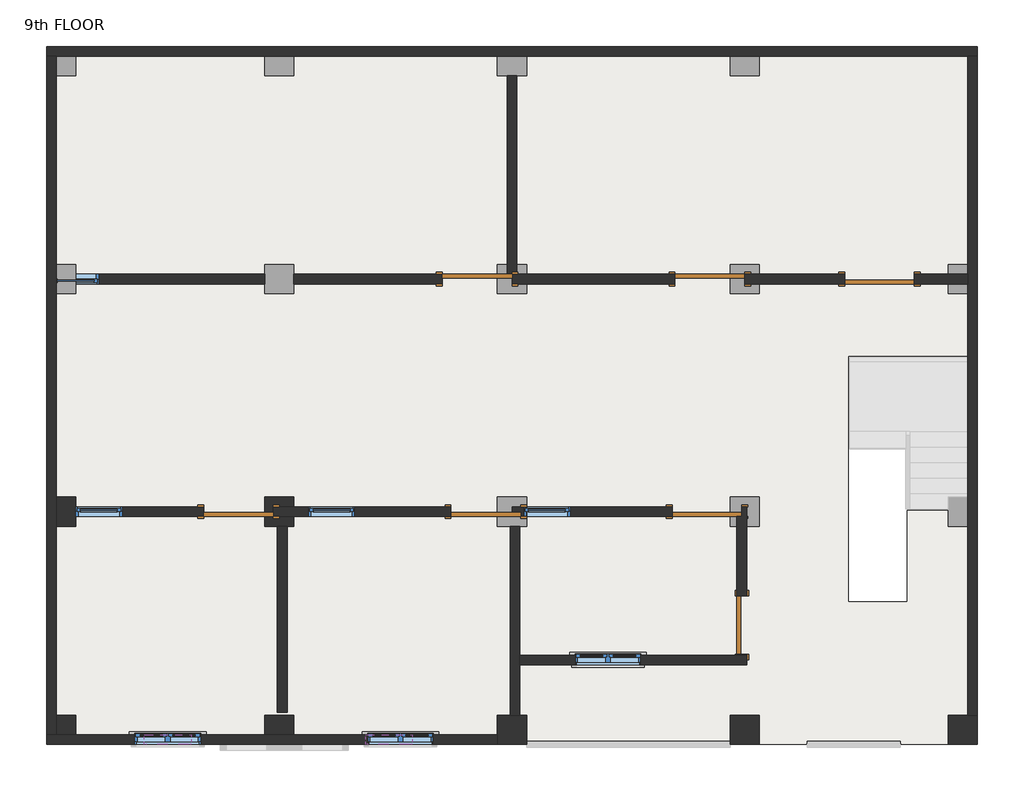
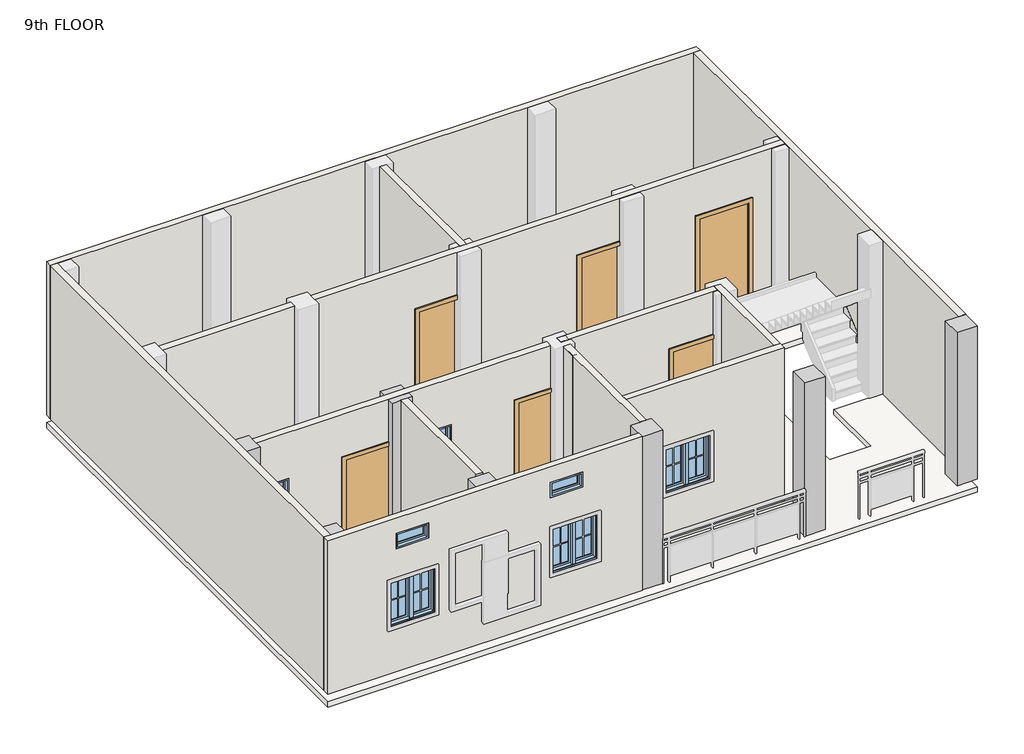
# One storey, part 1 of 2: 15 walls, 9 windows, 7 columns, 7 doors, 1 slab.
"""IFC4 building model written with IfcOpenShell, lengths in millimetres."""

from ifc_helpers import new_model, si_unit, frame, origin, place, context, project, spatial, polyline, outline, extrude, faceted_brep, transform, mapped, element, save
from components import door_e00f436c, door_a1797ceb, window_4c2727af, window_0bf3737e, window_78893e6c, window_0d9958e7

model = new_model("IFC4")

# Units and contexts
model_context = context("Model", 3, world=origin())
ifc_project = project(units=[si_unit("LENGTHUNIT", "METRE", prefix="MILLI")], contexts=[model_context])

# Site, building, storey
site = spatial("IfcSite", under=ifc_project)
building = spatial("IfcBuilding", under=site)
storey = spatial("IfcBuildingStorey", under=building, Name="9th FLOOR", Elevation=27279.6)

# Columns
placement = place(None, origin())
element("IfcColumn", 1, ObjectType="column family : column family", at=placement, inside=storey, context=model_context, shape_type="Brep", body=[
    faceted_brep([(-12576.097125, 2486.2065522, 27284.6), (-12957.097125, 2486.2065522, 27284.6), (-12957.097125, 2867.2065522, 27284.6), (-12576.097125, 2867.2065522, 27284.6), (-12576.097125, 2740.2065522, 27284.6), (-12842.797125, 2740.2065522, 27284.6), (-12842.797125, 2613.2065522, 27284.6), (-12576.097125, 2613.2065522, 27284.6), (-12576.097125, 2486.2065522, 30322.6), (-12576.097125, 2613.2065522, 30322.6), (-12957.097125, 2486.2065522, 30322.6), (-12957.097125, 2613.2065522, 30322.6), (-12957.097125, 2613.2065522, 29413.2), (-12957.097125, 2740.2065522, 29413.2), (-12957.097125, 2740.2065522, 30322.6), (-12957.097125, 2867.2065522, 30322.6), (-12576.097125, 2867.2065522, 30322.6), (-12842.797125, 2613.2065522, 29413.2), (-12842.797125, 2740.2065522, 29413.2), (-12576.097125, 2740.2065522, 30322.6)], [[[0, 1, 2, 3, 4, 5, 6, 7]], [[8, 0, 7, 9]], [[1, 0, 8, 10]], [[2, 1, 10, 11, 12, 13, 14, 15]], [[3, 2, 15, 16]], [[10, 8, 9, 11]], [[6, 17, 12, 11, 9, 7]], [[13, 18, 5, 4, 19, 14]], [[3, 16, 19, 4]], [[16, 15, 14, 19]], [[17, 18, 13, 12]], [[18, 17, 6, 5]]]),
])
element("IfcColumn", 2, ObjectType="column family : column family", at=placement, inside=storey, context=model_context, shape_type="SweptSolid", body=[
    extrude(outline(polyline([(-15433.597125, 2867.2065522), (-15433.597125, 2486.2065522), (-15687.597125, 2486.2065522), (-15687.597125, 2867.2065522), (-15433.597125, 2867.2065522)])), frame((0.0, 0.0, 27284.6), z_axis=(0.0, 0.0, 1.0), x_axis=(1.0, 0.0, 0.0)), (0.0, 0.0, 1.0), 3038.0),
])
element("IfcColumn", 3, ObjectType="column family : column family", at=placement, inside=storey, context=model_context, shape_type="SweptSolid", body=[
    extrude(outline(polyline([(-15433.597125, 9.7065522), (-15433.597125, -244.2934478), (-15687.597125, -244.2934478), (-15687.597125, 9.7065522), (-15433.597125, 9.7065522)])), frame((0.0, 0.0, 27284.6), z_axis=(0.0, 0.0, 1.0), x_axis=(1.0, 0.0, 0.0)), (0.0, 0.0, 1.0), 3038.0),
])
element("IfcColumn", 4, ObjectType="column family : column family", at=placement, inside=storey, context=model_context, shape_type="SweptSolid", body=[
    extrude(outline(polyline([(-3622.597125, 9.7065522), (-3622.597125, -371.2934478), (-4003.597125, -371.2934478), (-4003.597125, 9.7065522), (-3622.597125, 9.7065522)])), frame((0.0, 0.0, 27284.6), z_axis=(0.0, 0.0, 1.0), x_axis=(1.0, 0.0, 0.0)), (0.0, 0.0, 1.0), 3038.0),
])
element("IfcColumn", 5, ObjectType="column family : column family", at=placement, inside=storey, context=model_context, shape_type="SweptSolid", body=[
    extrude(outline(polyline([(-6480.097125, 9.7065522), (-6480.097125, -371.2934478), (-6861.097125, -371.2934478), (-6861.097125, 9.7065522), (-6480.097125, 9.7065522)])), frame((0.0, 0.0, 27284.6), z_axis=(0.0, 0.0, 1.0), x_axis=(1.0, 0.0, 0.0)), (0.0, 0.0, 1.0), 3038.0),
])
element("IfcColumn", 6, ObjectType="column family : column family", at=placement, inside=storey, context=model_context, shape_type="SweptSolid", body=[
    extrude(outline(polyline([(-9528.097125, 9.7065522), (-9528.097125, -371.2934478), (-9909.097125, -371.2934478), (-9909.097125, 9.7065522), (-9528.097125, 9.7065522)])), frame((0.0, 0.0, 27284.6), z_axis=(0.0, 0.0, 1.0), x_axis=(1.0, 0.0, 0.0)), (0.0, 0.0, 1.0), 3038.0),
])
element("IfcColumn", 7, ObjectType="column family : column family", at=placement, inside=storey, context=model_context, shape_type="SweptSolid", body=[
    extrude(outline(polyline([(-12957.097125, 9.7065522), (-12576.097125, 9.7065522), (-12576.097125, -244.2934478), (-12957.097125, -244.2934478), (-12957.097125, 9.7065522)])), frame((0.0, 0.0, 27284.6), z_axis=(0.0, 0.0, 1.0), x_axis=(1.0, 0.0, 0.0)), (0.0, 0.0, 1.0), 3038.0),
])

# Doors
door_shape = door_e00f436c(model_context)
element("IfcDoor", 8, ObjectType="Single-Flush : 30\" x 80\"", at=placement, inside=storey, context=model_context, shape_type="MappedRepresentation", body=[
    mapped(door_shape, transform((-6708.697125, 1190.8065522, 27279.6), x_axis=(0.0, -1.0, 0.0), y_axis=(1.0, 0.0, 0.0), z_axis=(0.0, 0.0, 1.0))),
])
door_2_shape = door_a1797ceb(model_context)
element("IfcDoor", 9, ObjectType="Single-Flush : 36\" x 84\"", at=placement, inside=storey, context=model_context, shape_type="MappedRepresentation", body=[
    mapped(door_2_shape, transform((-10175.797125, 5724.7065522, 27279.6), x_axis=(1.0, 0.0, 0.0), y_axis=(0.0, 1.0, 0.0), z_axis=(0.0, 0.0, 1.0))),
])
element("IfcDoor", 10, ObjectType="Single-Flush : 36\" x 84\"", at=placement, inside=storey, context=model_context, shape_type="MappedRepresentation", body=[
    mapped(door_2_shape, transform((-10061.497125, 2676.7065522, 27279.6), x_axis=(-1.0, 0.0, 0.0), y_axis=(0.0, -1.0, 0.0), z_axis=(0.0, 0.0, 1.0))),
])
element("IfcDoor", 11, ObjectType="Single-Flush : 36\" x 84\"", at=placement, inside=storey, context=model_context, shape_type="MappedRepresentation", body=[
    mapped(door_2_shape, transform((-13299.997125, 2676.7065522, 27279.6), x_axis=(-1.0, 0.0, 0.0), y_axis=(0.0, -1.0, 0.0), z_axis=(0.0, 0.0, 1.0))),
])
element("IfcDoor", 12, ObjectType="Single-Flush : 36\" x 84\"", at=placement, inside=storey, context=model_context, shape_type="MappedRepresentation", body=[
    mapped(door_2_shape, transform((-7127.797125, 5724.7065522, 27279.6), x_axis=(1.0, 0.0, 0.0), y_axis=(0.0, 1.0, 0.0), z_axis=(0.0, 0.0, 1.0))),
])
element("IfcDoor", 13, ObjectType="Single-Flush : 36\" x 84\"", at=placement, inside=storey, context=model_context, shape_type="MappedRepresentation", body=[
    mapped(door_2_shape, transform((-7165.897125, 2676.7065522, 27279.6), x_axis=(-1.0, 0.0, 0.0), y_axis=(0.0, -1.0, 0.0), z_axis=(0.0, 0.0, 1.0))),
])
element("IfcDoor", 14, ObjectType="Single-Flush : 36\" x 84\"", at=placement, inside=storey, context=model_context, shape_type="MappedRepresentation", body=[
    mapped(door_2_shape, transform((-4905.297125, 5724.7065522, 27279.6), x_axis=(-1.0, 0.0, 0.0), y_axis=(0.0, -1.0, 0.0), z_axis=(0.0, 0.0, 1.0))),
])

# Slab
element("IfcSlab", 15, ObjectType="Generic - 4\"", at=placement, inside=storey, context=model_context, shape_type="SweptSolid", body=[
    extrude(outline(polyline([(-3622.597125, 8772.7065522), (-3622.597125, -371.2934478), (-15814.597125, -371.2934478), (-15814.597125, 8772.7065522), (-3622.597125, 8772.7065522)]), holes=[polyline([(-3734.357125, 4711.0719226), (-5310.2646464, 4711.0719226), (-5310.2646464, 1502.3126957), (-4547.7736682, 1502.3126957), (-4547.7736682, 2699.911213), (-3734.357125, 2699.911213), (-3734.357125, 4711.0719226)])]), frame((0.0, 0.0, 27025.6), z_axis=(0.0, 0.0, 1.0), x_axis=(1.0, 0.0, 0.0)), (0.0, 0.0, 1.0), 101.6),
])

# Walls
element("IfcWall", 16, ObjectType="Generic - 5\"", at=placement, inside=storey, context=model_context, shape_type="Brep", body=[
    faceted_brep([(-15814.597125, 8645.7065522, 27279.6), (-15687.597125, 8645.7065522, 27279.6), (-3749.597125, 8645.7065522, 27279.6), (-3622.597125, 8645.7065522, 27279.6), (-3622.597125, 8645.7065522, 30327.6), (-3749.597125, 8645.7065522, 30327.6), (-15687.597125, 8645.7065522, 30327.6), (-15814.597125, 8645.7065522, 30327.6), (-15814.597125, 8772.7065522, 27279.6), (-15814.597125, 8772.7065522, 30327.6), (-3622.597125, 8772.7065522, 30327.6), (-3622.597125, 8772.7065522, 27279.6)], [[[0, 1, 2, 3, 4, 5, 6, 7]], [[8, 9, 10, 11]], [[3, 2, 1, 0, 8, 11]], [[7, 6, 5, 4, 10, 9]], [[4, 3, 11, 10]], [[0, 7, 9, 8]]]),
])
element("IfcWall", 17, ObjectType="Generic - 5\"", at=placement, inside=storey, context=model_context, shape_type="Brep", body=[
    faceted_brep([(-3749.597125, 8645.7065522, 27279.6), (-3749.597125, 5788.2065522, 27279.6), (-3749.597125, 5661.2065522, 27279.6), (-3749.597125, 9.7065522, 27279.6), (-3749.597125, 9.7065522, 30327.6), (-3749.597125, 5661.2065522, 30327.6), (-3749.597125, 5788.2065522, 30327.6), (-3749.597125, 8645.7065522, 30327.6), (-3622.597125, 8645.7065522, 27279.6), (-3622.597125, 8645.7065522, 30327.6), (-3622.597125, 9.7065522, 30327.6), (-3622.597125, 9.7065522, 30322.6), (-3622.597125, 9.7065522, 27284.6), (-3622.597125, 9.7065522, 27279.6)], [[[0, 1, 2, 3, 4, 5, 6, 7]], [[8, 9, 10, 11, 12, 13]], [[3, 2, 1, 0, 8, 13]], [[4, 3, 13, 12, 11, 10]], [[7, 6, 5, 4, 10, 9]], [[0, 7, 9, 8]]]),
])
element("IfcWall", 18, ObjectType="Generic - 5\"", at=placement, inside=storey, context=model_context, shape_type="Brep", body=[
    faceted_brep([(-9909.097125, -244.2934478, 27279.6), (-15687.597125, -244.2934478, 27279.6), (-15814.597125, -244.2934478, 27279.6), (-15814.597125, -244.2934478, 30327.6), (-15687.597125, -244.2934478, 30327.6), (-9909.097125, -244.2934478, 30327.6), (-13795.297125, -244.2934478, 29108.4), (-14658.897125, -244.2934478, 29108.4), (-14658.897125, -244.2934478, 28194.0), (-13795.297125, -244.2934478, 28194.0), (-10747.297125, -244.2934478, 29108.4), (-11610.897125, -244.2934478, 29108.4), (-11610.897125, -244.2934478, 28194.0), (-10747.297125, -244.2934478, 28194.0), (-13922.297125, -244.2934478, 30022.8), (-14531.897125, -244.2934478, 30022.8), (-14531.897125, -244.2934478, 29718.0), (-13922.297125, -244.2934478, 29718.0), (-11026.697125, -244.2934478, 30022.8), (-11636.297125, -244.2934478, 30022.8), (-11636.297125, -244.2934478, 29718.0), (-11026.697125, -244.2934478, 29718.0), (-9909.097125, -371.2934478, 27279.6), (-9909.097125, -371.2934478, 27284.6), (-9909.097125, -371.2934478, 30322.6), (-9909.097125, -371.2934478, 30327.6), (-15814.597125, -371.2934478, 30327.6), (-15814.597125, -371.2934478, 27279.6), (-13795.297125, -371.2934478, 29108.4), (-13795.297125, -371.2934478, 28194.0), (-14658.897125, -371.2934478, 28194.0), (-14658.897125, -371.2934478, 29108.4), (-10747.297125, -371.2934478, 29108.4), (-10747.297125, -371.2934478, 28194.0), (-11610.897125, -371.2934478, 28194.0), (-11610.897125, -371.2934478, 29108.4), (-13922.297125, -371.2934478, 30022.8), (-13922.297125, -371.2934478, 29718.0), (-14531.897125, -371.2934478, 29718.0), (-14531.897125, -371.2934478, 30022.8), (-11026.697125, -371.2934478, 30022.8), (-11026.697125, -371.2934478, 29718.0), (-11636.297125, -371.2934478, 29718.0), (-11636.297125, -371.2934478, 30022.8)], [[[0, 1, 2, 3, 4, 5], [6, 7, 8, 9], [10, 11, 12, 13], [14, 15, 16, 17], [18, 19, 20, 21]], [[22, 23, 24, 25, 26, 27], [28, 29, 30, 31], [32, 33, 34, 35], [36, 37, 38, 39], [40, 41, 42, 43]], [[2, 1, 0, 22, 27]], [[5, 4, 3, 26, 25]], [[0, 5, 25, 24, 23, 22]], [[3, 2, 27, 26]], [[29, 28, 6, 9]], [[30, 29, 9, 8]], [[31, 30, 8, 7]], [[28, 31, 7, 6]], [[33, 32, 10, 13]], [[34, 33, 13, 12]], [[35, 34, 12, 11]], [[32, 35, 11, 10]], [[37, 36, 14, 17]], [[38, 37, 17, 16]], [[39, 38, 16, 15]], [[36, 39, 15, 14]], [[41, 40, 18, 21]], [[42, 41, 21, 20]], [[43, 42, 20, 19]], [[40, 43, 19, 18]]]),
])
element("IfcWall", 19, ObjectType="Generic - 5\"", at=placement, inside=storey, context=model_context, shape_type="Brep", body=[
    faceted_brep([(-15687.597125, -244.2934478, 27279.6), (-15687.597125, 8645.7065522, 27279.6), (-15687.597125, 8645.7065522, 27284.6), (-15687.597125, 8645.7065522, 30322.6), (-15687.597125, 8645.7065522, 30327.6), (-15687.597125, -244.2934478, 30327.6), (-15687.597125, -244.2934478, 30322.6), (-15687.597125, -244.2934478, 27284.6), (-15814.597125, -244.2934478, 27279.6), (-15814.597125, -244.2934478, 30327.6), (-15814.597125, 8645.7065522, 30327.6), (-15814.597125, 8645.7065522, 27279.6)], [[[0, 1, 2, 3, 4, 5, 6, 7]], [[8, 9, 10, 11]], [[1, 0, 8, 11]], [[5, 4, 10, 9]], [[4, 3, 2, 1, 11, 10]], [[0, 7, 6, 5, 9, 8]]]),
])
element("IfcWall", 20, ObjectType="Generic - 5\"", at=placement, inside=storey, context=model_context, shape_type="SweptSolid", body=[
    extrude(outline(polyline([(27279.6, -15433.597125), (27279.6, -12957.097125), (30327.6, -12957.097125), (30327.6, -15433.597125), (29413.2, -15433.597125), (29413.2, -15128.797125), (27584.4, -15128.797125), (27584.4, -15433.597125), (27279.6, -15433.597125)])), frame((0.0, 5661.2065522, 0.0), z_axis=(0.0, 1.0, 0.0), x_axis=(0.0, 0.0, 1.0)), (0.0, 0.0, 1.0), 127.0),
])
element("IfcWall", 21, ObjectType="Generic - 5\"", at=placement, inside=storey, context=model_context, shape_type="Brep", body=[
    faceted_brep([(-9782.097125, 8391.7065522, 27279.6), (-9782.097125, 5788.2065522, 27279.6), (-9782.097125, 5788.2065522, 27284.6), (-9782.097125, 5788.2065522, 29413.2), (-9782.097125, 5788.2065522, 30322.6), (-9782.097125, 5788.2065522, 30327.6), (-9782.097125, 8391.7065522, 30327.6), (-9655.097125, 8391.7065522, 27279.6), (-9655.097125, 8391.7065522, 30327.6), (-9655.097125, 5788.2065522, 30327.6), (-9655.097125, 5788.2065522, 30322.6), (-9655.097125, 5788.2065522, 27284.6), (-9655.097125, 5788.2065522, 27279.6), (-9718.597125, 5788.2065522, 27279.6)], [[[0, 1, 2, 3, 4, 5, 6]], [[7, 8, 9, 10, 11, 12]], [[1, 0, 7, 12, 13]], [[6, 5, 9, 8]], [[0, 6, 8, 7]], [[5, 4, 3, 2, 1, 13, 12, 11, 10, 9]]]),
])
element("IfcWall", 22, ObjectType="Generic - 5\"", at=placement, inside=storey, context=model_context, shape_type="Brep", body=[
    faceted_brep([(-6670.597125, 5661.2065522, 27279.6), (-5362.497125, 5661.2065522, 27279.6), (-5362.497125, 5661.2065522, 29413.2), (-4448.097125, 5661.2065522, 29413.2), (-4448.097125, 5661.2065522, 27279.6), (-3749.597125, 5661.2065522, 27279.6), (-3749.597125, 5661.2065522, 27284.6), (-3749.597125, 5661.2065522, 30322.6), (-3749.597125, 5661.2065522, 30327.6), (-12576.097125, 5661.2065522, 30327.6), (-12576.097125, 5661.2065522, 27279.6), (-10632.997125, 5661.2065522, 27279.6), (-10632.997125, 5661.2065522, 29413.2), (-9909.097125, 5661.2065522, 29413.2), (-9718.597125, 5661.2065522, 29413.2), (-9718.597125, 5661.2065522, 27284.6), (-9718.597125, 5661.2065522, 27279.6), (-7584.997125, 5661.2065522, 27279.6), (-7584.997125, 5661.2065522, 29413.2), (-6861.097125, 5661.2065522, 29413.2), (-6670.597125, 5661.2065522, 29413.2), (-6670.597125, 5661.2065522, 27284.6), (-5362.497125, 5788.2065522, 29413.2), (-5362.497125, 5788.2065522, 27279.6), (-6670.597125, 5788.2065522, 27279.6), (-6670.597125, 5788.2065522, 27284.6), (-6670.597125, 5788.2065522, 29413.2), (-6861.097125, 5788.2065522, 29413.2), (-7584.997125, 5788.2065522, 29413.2), (-7584.997125, 5788.2065522, 27279.6), (-9655.097125, 5788.2065522, 27279.6), (-9718.597125, 5788.2065522, 27279.6), (-9718.597125, 5788.2065522, 27284.6), (-9718.597125, 5788.2065522, 29413.2), (-9782.097125, 5788.2065522, 29413.2), (-9909.097125, 5788.2065522, 29413.2), (-10632.997125, 5788.2065522, 29413.2), (-10632.997125, 5788.2065522, 27279.6), (-12576.097125, 5788.2065522, 27279.6), (-12576.097125, 5788.2065522, 30327.6), (-9782.097125, 5788.2065522, 30327.6), (-9655.097125, 5788.2065522, 30327.6), (-3749.597125, 5788.2065522, 30327.6), (-3749.597125, 5788.2065522, 30322.6), (-3749.597125, 5788.2065522, 27284.6), (-3749.597125, 5788.2065522, 27279.6), (-4448.097125, 5788.2065522, 27279.6), (-4448.097125, 5788.2065522, 29413.2)], [[[0, 1, 2, 3, 4, 5, 6, 7, 8, 9, 10, 11, 12, 13, 14, 15, 16, 17, 18, 19, 20, 21]], [[22, 23, 24, 25, 26, 27, 28, 29, 30, 31, 32, 33, 34, 35, 36, 37, 38, 39, 40, 41, 42, 43, 44, 45, 46, 47]], [[11, 10, 38, 37]], [[17, 16, 31, 30, 29]], [[46, 45, 5, 4]], [[24, 23, 1, 0]], [[9, 8, 42, 41, 40, 39]], [[10, 9, 39, 38]], [[8, 7, 6, 5, 45, 44, 43, 42]], [[33, 32, 31, 16, 15, 14]], [[36, 35, 34, 33, 14, 13, 12]], [[37, 36, 12, 11]], [[26, 25, 24, 0, 21, 20]], [[28, 27, 26, 20, 19, 18]], [[29, 28, 18, 17]], [[2, 1, 23, 22]], [[3, 2, 22, 47]], [[4, 3, 47, 46]]]),
])
element("IfcWall", 23, ObjectType="Generic - 5\"", at=placement, inside=storey, context=model_context, shape_type="Brep", body=[
    faceted_brep([(-14823.997125, 2613.2065522, 27584.4), (-15433.597125, 2613.2065522, 27584.4), (-15433.597125, 2613.2065522, 27279.6), (-13757.197125, 2613.2065522, 27279.6), (-13757.197125, 2613.2065522, 29413.2), (-12957.097125, 2613.2065522, 29413.2), (-12842.797125, 2613.2065522, 29413.2), (-12842.797125, 2613.2065522, 27284.6), (-12842.797125, 2613.2065522, 27279.6), (-10518.697125, 2613.2065522, 27279.6), (-10518.697125, 2613.2065522, 29413.2), (-9909.097125, 2613.2065522, 29413.2), (-9909.097125, 2613.2065522, 30327.6), (-15433.597125, 2613.2065522, 30327.6), (-15433.597125, 2613.2065522, 29413.2), (-14823.997125, 2613.2065522, 29413.2), (-12385.597125, 2613.2065522, 29413.2), (-11775.997125, 2613.2065522, 29413.2), (-11775.997125, 2613.2065522, 27584.4), (-12385.597125, 2613.2065522, 27584.4), (-15433.597125, 2740.2065522, 27279.6), (-15433.597125, 2740.2065522, 27584.4), (-14823.997125, 2740.2065522, 27584.4), (-14823.997125, 2740.2065522, 29413.2), (-15433.597125, 2740.2065522, 29413.2), (-15433.597125, 2740.2065522, 30327.6), (-9909.097125, 2740.2065522, 30327.6), (-9909.097125, 2740.2065522, 29413.2), (-10518.697125, 2740.2065522, 29413.2), (-10518.697125, 2740.2065522, 27279.6), (-12842.797125, 2740.2065522, 27279.6), (-12842.797125, 2740.2065522, 27284.6), (-12842.797125, 2740.2065522, 29413.2), (-12957.097125, 2740.2065522, 29413.2), (-13757.197125, 2740.2065522, 29413.2), (-13757.197125, 2740.2065522, 27279.6), (-12385.597125, 2740.2065522, 29413.2), (-12385.597125, 2740.2065522, 27584.4), (-11775.997125, 2740.2065522, 27584.4), (-11775.997125, 2740.2065522, 29413.2)], [[[0, 1, 2, 3, 4, 5, 6, 7, 8, 9, 10, 11, 12, 13, 14, 15], [16, 17, 18, 19]], [[20, 21, 22, 23, 24, 25, 26, 27, 28, 29, 30, 31, 32, 33, 34, 35], [36, 37, 38, 39]], [[30, 29, 9, 8]], [[20, 35, 3, 2]], [[26, 12, 11, 27]], [[13, 12, 26, 25]], [[14, 13, 25, 24]], [[2, 1, 21, 20]], [[28, 10, 9, 29]], [[10, 28, 27, 11]], [[4, 3, 35, 34]], [[6, 5, 4, 34, 33, 32]], [[8, 7, 6, 32, 31, 30]], [[22, 21, 1, 0]], [[23, 22, 0, 15]], [[24, 23, 15, 14]], [[37, 36, 16, 19]], [[38, 37, 19, 18]], [[39, 38, 18, 17]], [[36, 39, 17, 16]]]),
])
element("IfcWall", 24, ObjectType="Generic - 5\"", at=placement, inside=storey, context=model_context, shape_type="Brep", body=[
    faceted_brep([(-9616.997125, 9.7065522, 27279.6), (-9616.997125, 670.1065522, 27279.6), (-9616.997125, 797.1065522, 27279.6), (-9616.997125, 2486.2065522, 27279.6), (-9616.997125, 2486.2065522, 30327.6), (-9616.997125, 797.1065522, 30327.6), (-9616.997125, 670.1065522, 30327.6), (-9616.997125, 9.7065522, 30327.6), (-9743.997125, 9.7065522, 27279.6), (-9743.997125, 9.7065522, 30327.6), (-9743.997125, 2486.2065522, 30327.6), (-9743.997125, 2486.2065522, 27279.6)], [[[0, 1, 2, 3, 4, 5, 6, 7]], [[8, 9, 10, 11]], [[3, 2, 1, 0, 8, 11]], [[4, 3, 11, 10]], [[7, 6, 5, 4, 10, 9]], [[0, 7, 9, 8]]]),
])
element("IfcWall", 25, ObjectType="Generic - 5\"", at=placement, inside=storey, context=model_context, shape_type="SweptSolid", body=[
    extrude(outline(polyline([(-9743.997125, 2181.4065522), (-9743.997125, 2486.2065522), (-9616.997125, 2486.2065522), (-9616.997125, 2181.4065522), (-9743.997125, 2181.4065522)])), frame((0.0, 0.0, 27279.6), z_axis=(0.0, 0.0, 1.0), x_axis=(1.0, 0.0, 0.0)), (0.0, 0.0, 1.0), 3048.0),
])
element("IfcWall", 26, ObjectType="Generic - 5\"", at=placement, inside=storey, context=model_context, shape_type="Brep", body=[
    faceted_brep([(-6772.197125, 2613.2065522, 30327.6), (-9718.597125, 2613.2065522, 30327.6), (-9718.597125, 2613.2065522, 30322.6), (-9718.597125, 2613.2065522, 27284.6), (-9718.597125, 2613.2065522, 27279.6), (-7623.097125, 2613.2065522, 27279.6), (-7623.097125, 2613.2065522, 29413.2), (-6861.097125, 2613.2065522, 29413.2), (-6772.197125, 2613.2065522, 29413.2), (-6772.197125, 2613.2065522, 30322.6), (-9566.197125, 2613.2065522, 29413.2), (-9528.097125, 2613.2065522, 29413.2), (-8956.597125, 2613.2065522, 29413.2), (-8956.597125, 2613.2065522, 27584.4), (-9528.097125, 2613.2065522, 27584.4), (-9566.197125, 2613.2065522, 27584.4), (-9718.597125, 2740.2065522, 30327.6), (-6772.197125, 2740.2065522, 30327.6), (-6772.197125, 2740.2065522, 29413.2), (-6861.097125, 2740.2065522, 29413.2), (-7623.097125, 2740.2065522, 29413.2), (-7623.097125, 2740.2065522, 27279.6), (-9718.597125, 2740.2065522, 27279.6), (-9718.597125, 2740.2065522, 27284.6), (-9718.597125, 2740.2065522, 30322.6), (-9566.197125, 2740.2065522, 29413.2), (-9566.197125, 2740.2065522, 27584.4), (-9528.097125, 2740.2065522, 27584.4), (-8956.597125, 2740.2065522, 27584.4), (-8956.597125, 2740.2065522, 29413.2), (-9528.097125, 2740.2065522, 29413.2)], [[[0, 1, 2, 3, 4, 5, 6, 7, 8, 9], [10, 11, 12, 13, 14, 15]], [[16, 17, 18, 19, 20, 21, 22, 23, 24], [25, 26, 27, 28, 29, 30]], [[4, 22, 21, 5]], [[1, 0, 17, 16]], [[4, 3, 2, 1, 16, 24, 23, 22]], [[26, 25, 10, 15]], [[28, 27, 26, 15, 14, 13]], [[29, 28, 13, 12]], [[25, 30, 29, 12, 11, 10]], [[20, 6, 5, 21]], [[6, 20, 19, 18, 8, 7]], [[17, 0, 9, 8, 18]]]),
])
element("IfcWall", 27, ObjectType="Generic - 5\"", at=placement, inside=storey, context=model_context, shape_type="Brep", body=[
    faceted_brep([(-6645.197125, 797.1065522, 27279.6), (-6645.197125, 809.8065522, 27279.6), (-6645.197125, 809.8065522, 29311.6), (-6645.197125, 1571.8065522, 29311.6), (-6645.197125, 1571.8065522, 27279.6), (-6645.197125, 2740.2065522, 27279.6), (-6645.197125, 2740.2065522, 27284.6), (-6645.197125, 2740.2065522, 30322.6), (-6645.197125, 2740.2065522, 30327.6), (-6645.197125, 797.1065522, 30327.6), (-6772.197125, 809.8065522, 29311.6), (-6772.197125, 809.8065522, 27279.6), (-6772.197125, 797.1065522, 27279.6), (-6772.197125, 797.1065522, 30327.6), (-6772.197125, 2613.2065522, 30327.6), (-6772.197125, 2740.2065522, 30327.6), (-6772.197125, 2740.2065522, 29413.2), (-6772.197125, 2613.2065522, 29413.2), (-6772.197125, 2613.2065522, 27284.6), (-6772.197125, 2613.2065522, 27279.6), (-6772.197125, 1571.8065522, 27279.6), (-6772.197125, 1571.8065522, 29311.6), (-6708.697125, 2613.2065522, 27279.6), (-6708.697125, 2740.2065522, 27279.6), (-6708.697125, 2613.2065522, 29413.2), (-6708.697125, 2613.2065522, 27284.6), (-6708.697125, 2740.2065522, 29413.2), (-6708.697125, 2740.2065522, 27284.6)], [[[0, 1, 2, 3, 4, 5, 6, 7, 8, 9]], [[10, 11, 12, 13, 14, 15, 16, 17, 18, 19, 20, 21]], [[20, 19, 22, 23, 5, 4]], [[12, 11, 1, 0]], [[9, 8, 15, 14, 13]], [[24, 25, 22, 19, 18, 17]], [[26, 24, 17, 16]], [[22, 25, 24, 26, 27, 23]], [[8, 7, 6, 5, 23, 27, 26, 16, 15]], [[0, 9, 13, 12]], [[2, 1, 11, 10]], [[3, 2, 10, 21]], [[4, 3, 21, 20]]]),
])
element("IfcWall", 28, ObjectType="Generic - 5\"", at=placement, inside=storey, context=model_context, shape_type="Brep", body=[
    faceted_brep([(-9718.597125, 2613.2065522, 27279.6), (-9566.197125, 2613.2065522, 27279.6), (-9566.197125, 2613.2065522, 27584.4), (-9566.197125, 2613.2065522, 29413.2), (-9566.197125, 2613.2065522, 30327.6), (-9718.597125, 2613.2065522, 30327.6), (-9718.597125, 2613.2065522, 30322.6), (-9718.597125, 2613.2065522, 27284.6), (-9718.597125, 2740.2065522, 27279.6), (-9718.597125, 2740.2065522, 27284.6), (-9718.597125, 2740.2065522, 30322.6), (-9718.597125, 2740.2065522, 30327.6), (-9566.197125, 2740.2065522, 30327.6), (-9566.197125, 2740.2065522, 29413.2), (-9566.197125, 2740.2065522, 27584.4), (-9566.197125, 2740.2065522, 27279.6)], [[[0, 1, 2, 3, 4, 5, 6, 7]], [[8, 9, 10, 11, 12, 13, 14, 15]], [[1, 0, 8, 15]], [[4, 3, 2, 1, 15, 14, 13, 12]], [[5, 4, 12, 11]], [[0, 7, 6, 5, 11, 10, 9, 8]]]),
])
element("IfcWall", 29, ObjectType="Generic - 5\"", at=placement, inside=storey, context=model_context, shape_type="SweptSolid", body=[
    extrude(outline(polyline([(-12791.997125, 47.8065522), (-12791.997125, 2486.2065522), (-12664.997125, 2486.2065522), (-12664.997125, 47.8065522), (-12791.997125, 47.8065522)])), frame((0.0, 0.0, 27279.6), z_axis=(0.0, 0.0, 1.0), x_axis=(1.0, 0.0, 0.0)), (0.0, 0.0, 1.0), 3048.0),
])
element("IfcWall", 30, ObjectType="Generic - 5\"", at=placement, inside=storey, context=model_context, shape_type="Brep", body=[
    faceted_brep([(-9616.997125, 670.1065522, 27279.6), (-6645.197125, 670.1065522, 27279.6), (-6645.197125, 670.1065522, 30327.6), (-9616.997125, 670.1065522, 30327.6), (-8029.497125, 670.1065522, 29108.4), (-8029.497125, 670.1065522, 28194.0), (-8893.097125, 670.1065522, 28194.0), (-8893.097125, 670.1065522, 29108.4), (-9616.997125, 797.1065522, 27279.6), (-9616.997125, 797.1065522, 30327.6), (-6772.197125, 797.1065522, 30327.6), (-6645.197125, 797.1065522, 30327.6), (-6645.197125, 797.1065522, 27279.6), (-6772.197125, 797.1065522, 27279.6), (-8029.497125, 797.1065522, 29108.4), (-8893.097125, 797.1065522, 29108.4), (-8893.097125, 797.1065522, 28194.0), (-8029.497125, 797.1065522, 28194.0)], [[[0, 1, 2, 3], [4, 5, 6, 7]], [[8, 9, 10, 11, 12, 13], [14, 15, 16, 17]], [[1, 0, 8, 13, 12]], [[3, 2, 11, 10, 9]], [[0, 3, 9, 8]], [[2, 1, 12, 11]], [[5, 4, 14, 17]], [[6, 5, 17, 16]], [[7, 6, 16, 15]], [[4, 7, 15, 14]]]),
])

# Windows
window_shape = window_4c2727af(model_context)
element("IfcWindow", 31, ObjectType="Fixed : 24\" x 12\"", at=placement, inside=storey, context=model_context, shape_type="MappedRepresentation", body=[
    mapped(window_shape, transform((-14188.997125, -307.7934478, 28803.6), x_axis=(1.0, 0.0, 0.0), y_axis=(0.0, 1.0, 0.0), z_axis=(0.0, 0.0, 1.0))),
])
element("IfcWindow", 32, ObjectType="Fixed : 24\" x 12\"", at=placement, inside=storey, context=model_context, shape_type="MappedRepresentation", body=[
    mapped(window_shape, transform((-11293.397125, -307.7934478, 28803.6), x_axis=(1.0, 0.0, 0.0), y_axis=(0.0, 1.0, 0.0), z_axis=(0.0, 0.0, 1.0))),
])
window_2_shape = window_0bf3737e(model_context)
element("IfcWindow", 33, ObjectType="Fixed : 24\" x 72\"", at=placement, inside=storey, context=model_context, shape_type="MappedRepresentation", body=[
    mapped(window_2_shape, transform((-15471.697125, 5724.7065522, 27279.6), x_axis=(-1.0, 0.0, 0.0), y_axis=(0.0, -1.0, 0.0), z_axis=(0.0, 0.0, 1.0))),
])
window_3_shape = window_78893e6c(model_context)
element("IfcWindow", 34, ObjectType="Fixed : 24\" x 72\"", at=placement, inside=storey, context=model_context, shape_type="MappedRepresentation", body=[
    mapped(window_3_shape, transform((-15166.897125, 2676.7065522, 27279.6), x_axis=(-1.0, 0.0, 0.0), y_axis=(0.0, -1.0, 0.0), z_axis=(0.0, 0.0, 1.0))),
])
element("IfcWindow", 35, ObjectType="Fixed : 24\" x 72\"", at=placement, inside=storey, context=model_context, shape_type="MappedRepresentation", body=[
    mapped(window_3_shape, transform((-12118.897125, 2676.7065522, 27279.6), x_axis=(-1.0, 0.0, 0.0), y_axis=(0.0, -1.0, 0.0), z_axis=(0.0, 0.0, 1.0))),
])
element("IfcWindow", 36, ObjectType="Fixed : 24\" x 72\"", at=placement, inside=storey, context=model_context, shape_type="MappedRepresentation", body=[
    mapped(window_3_shape, transform((-9299.497125, 2676.7065522, 27279.6), x_axis=(-1.0, 0.0, 0.0), y_axis=(0.0, -1.0, 0.0), z_axis=(0.0, 0.0, 1.0))),
])
window_4_shape = window_0d9958e7(model_context)
element("IfcWindow", 37, ObjectType="Window-Casement-Double : 34\" x 36\"", at=placement, inside=storey, context=model_context, shape_type="MappedRepresentation", body=[
    mapped(window_4_shape, transform((-14227.097125, -307.7934478, 27279.6), x_axis=(1.0, 0.0, 0.0), y_axis=(0.0, 1.0, 0.0), z_axis=(0.0, 0.0, 1.0))),
])
element("IfcWindow", 38, ObjectType="Window-Casement-Double : 34\" x 36\"", at=placement, inside=storey, context=model_context, shape_type="MappedRepresentation", body=[
    mapped(window_4_shape, transform((-11179.097125, -307.7934478, 27279.6), x_axis=(1.0, 0.0, 0.0), y_axis=(0.0, 1.0, 0.0), z_axis=(0.0, 0.0, 1.0))),
])
element("IfcWindow", 39, ObjectType="Window-Casement-Double : 34\" x 36\"", at=placement, inside=storey, context=model_context, shape_type="MappedRepresentation", body=[
    mapped(window_4_shape, transform((-8461.297125, 733.6065522, 27279.6), x_axis=(1.0, 0.0, 0.0), y_axis=(0.0, 1.0, 0.0), z_axis=(0.0, 0.0, 1.0))),
])

save(model, "model.ifc")

# Revit data of these elements
# Type "column family : column family"
#   w2 [instance default] = 0' - 9.88189"
#   w1 [instance default] = 0' - 9.01575"
#   Depth = 1' - 11.62205"
#   Width = 1' - 11.62205"
# Type "Single-Flush : 30\" x 80\""
#   Type Mark = "5"
#   Construction Type Id = "MDOOR"
#   Assembly Code = "C1020"
#   Analytic Construction = "Metal"
#   Thickness = 0' - 2"
#   Heat Transfer Coefficient (U) = 0.651978 BTU/(h·ft²·°F)
#   Height = 6' - 8"
#   Trim Projection Ext = 0' - 1"
#   Trim Projection Int = 0' - 1"
#   Trim Width = 0' - 3"
#   Width = 2' - 6"
#   Define Thermal Properties by = 1
#   Define Thermal Properties by = 1
#   Door Material = Door - Panel
#   Frame Material = Door - Frame
#   Visual Light Transmittance = 0
#   Solar Heat Gain Coefficient = 0
#   Function = (empty or 0)
#   Wall Closure = (empty or 0)
# Type "Single-Flush : 36\" x 84\""
#   Type Mark = "1"
#   Construction Type Id = "MDOOR"
#   Assembly Code = "C1020"
#   Analytic Construction = "Metal"
#   Thickness = 0' - 2"
#   Heat Transfer Coefficient (U) = 0.651978 BTU/(h·ft²·°F)
#   Height = 7' - 0"
#   Trim Projection Ext = 0' - 1"
#   Trim Projection Int = 0' - 1"
#   Trim Width = 0' - 3"
#   Width = 3' - 0"
#   Define Thermal Properties by = 1
#   Define Thermal Properties by = 1
#   Door Material = Door - Panel
#   Frame Material = Door - Frame
#   Visual Light Transmittance = 0
#   Solar Heat Gain Coefficient = 0
#   Function = (empty or 0)
#   Wall Closure = (empty or 0)
# Type "Generic - 4\""
#   Assembly Code = "B1010"
#   Function = 0
#   Layers, outside or top first: 0' - 4" no material (function 1)
# Type "Generic - 5\""
#   Assembly Code = "B2010"
#   Layers, outside or top first: 0' - 5" no material (function 1)
# Type "Fixed : 24\" x 12\""
#   Type Mark = "4"
#   Construction Type Id = "GSP4R"
#   Assembly Code = "B2020100"
#   Analytic Construction = "1/8 in Pilkington single glazing"
#   Visual Light Transmittance = 0.9
#   Solar Heat Gain Coefficient = 0.78
#   Heat Transfer Coefficient (U) = 0.6496 BTU/(h·ft²·°F)
#   Height = 1' - 0"
#   Default Sill Height = 3' - 0"
#   Width = 2' - 0"
#   Window Inset = 0' - 0 3/4"
#   Define Thermal Properties by = 1
#   Define Thermal Properties by = 1
#   Glass Pane Material = Glass
#   Sash Material = Sash
#   Wall Closure = (empty or 0)
# Type "Fixed : 24\" x 72\""
#   Type Mark = "7"
#   Construction Type Id = "GSP4R"
#   Assembly Code = "B2020100"
#   Analytic Construction = "1/8 in Pilkington single glazing"
#   Visual Light Transmittance = 0.9
#   Solar Heat Gain Coefficient = 0.78
#   Heat Transfer Coefficient (U) = 0.6496 BTU/(h·ft²·°F)
#   Height = 6' - 0"
#   Default Sill Height = 1' - 0"
#   Width = 2' - 0"
#   Window Inset = 0' - 0 3/4"
#   Define Thermal Properties by = 1
#   Define Thermal Properties by = 1
#   Glass Pane Material = Glass
#   Sash Material = Sash
#   Wall Closure = (empty or 0)
# Type "Window-Casement-Double : 34\" x 36\""
#   Type Mark = "14"
#   Fire Rating = "0.5h"
#   Assembly Code = "B2020100"
#   Analytic Construction = "Double glazing - domestic"
#   Frame Extension [instance default] = 0' - 0 1/4"
#   Window Inset [instance default] = 0' - 0"
#   Wall Thickness [instance default] = 0' - 6"
#   Interior Wall Closure [instance default] = 0' - 2 1/4"
#   Half Width = 1' - 5"
#   Visual Light Transmittance = 0.81
#   Thermal Resistance (R) = 1.8146 (h·ft²·°F)/BTU
#   Solar Heat Gain Coefficient = 0.76
#   Rough Width = 2' - 10 1/2"
#   Rough Height = 3' - 0 1/2"
#   Height = 3' - 0"
#   Heat Transfer Coefficient (U) = 0.5511 BTU/(h·ft²·°F)
#   Exterior Wall Closure [instance default] = 0' - 1 1/4"
#   Extension Jamb [instance default] = 0' - 2 1/4"
#   Default Sill Height = 3' - 0"
#   Width = 2' - 10"
#   Define Thermal Properties by = 0
#   Muntin Visibility = yes
#   Interior Trim Visibility [instance default] = yes
#   Exterior Trim Visibility [instance default] = yes
#   Extension Jamb Visibility [instance default] = yes
#   Interior Trim Material = Wood - Stained
#   Muntin Pattern = Muntin Pattern_2x2 : Muntin Pattern_2x2
#   Interior Trim = Trim-Window-Interior-Flat : Picture Frame
#   Interior Frame Material = Wood - Stained
#   Glass Panel Material = Glass
#   Exterior Trim Material = Clad - White
#   Exterior Trim = Trim-Window-Exterior-Flat : with Sill
#   Exterior Frame Material = Clad - White
#   Wall Closure = (empty or 0)
# Element 1 (IfcColumn, "column family : column family")
#   w2 = 1' - 3"
#   w1 = 1' - 3"
#   Phase Created = New Construction
#   Materials on its faces: "Default Wall", "inside wall"
# Element 2 (IfcColumn, "column family : column family")
#   w2 = 1' - 3"
#   w1 = 0' - 10"
#   Phase Created = New Construction
#   Materials on its faces: "inside wall", "Default Wall"
# Elements 3, 7 (IfcColumn, "column family : column family")
#   w2 = 1' - 3"
#   w1 = 1' - 3"
#   Phase Created = New Construction
#   Materials on its faces: "Default Wall"
# Element 4 (IfcColumn, "column family : column family")
#   w2 = 1' - 3"
#   w1 = 1' - 3"
#   Phase Created = New Construction
#   Materials on its faces: "Clad - White", "Default Wall"
# Element 5 (IfcColumn, "column family : column family")
#   w2 = 1' - 3"
#   w1 = 1' - 3"
#   Phase Created = New Construction
#   Materials on its faces: "out side wall"
# Element 6 (IfcColumn, "column family : column family")
#   w2 = 1' - 3"
#   w1 = 1' - 3"
#   Phase Created = New Construction
#   Materials on its faces: "out side wall", "Default Wall"
# Element 8 (IfcDoor, "Single-Flush : 30\" x 80\"")
#   Phase Created = New Construction
#   Materials on its faces: "Door - Frame", "Door - Panel"
# Elements 9, 10, 11, 12, 13, 14 (IfcDoor, "Single-Flush : 36\" x 84\"")
#   Phase Created = New Construction
#   Materials on its faces: "Door - Frame", "Door - Panel"
# Element 15 (IfcSlab, "Generic - 4\"")
#   Height Offset From Level = -0' - 6"
#   Phase Created = New Construction
#   Materials on its faces: "Default Floor", "Clad - White", "floor"
# Element 16 (IfcWall, "Generic - 5\"")
#   Top Offset = 0' - 0"
#   Base Offset = 0' - 0"
#   wall height = 10' - 0"
#   Phase Created = New Construction
#   Base Constraint = 9th FLOOR
#   Top Constraint = 10th FLOOR
#   Materials on its faces: "Default Wall", "Clad - White"
# Element 17 (IfcWall, "Generic - 5\"")
#   Top Offset = 0' - 0"
#   Base Offset = 0' - 0"
#   wall height = 10' - 0"
#   Phase Created = New Construction
#   Base Constraint = 9th FLOOR
#   Top Constraint = 10th FLOOR
#   Materials on its faces: "Default Wall", "grey", "Clad - White"
# Element 18 (IfcWall, "Generic - 5\"")
#   Top Offset = 0' - 0"
#   Base Offset = 0' - 0"
#   wall height = 10' - 0"
#   Phase Created = New Construction
#   Base Constraint = 9th FLOOR
#   Top Constraint = 10th FLOOR
#   Materials on its faces: "Default Wall", "out side wall", "Clad - White"
# Element 19 (IfcWall, "Generic - 5\"")
#   Top Offset = 0' - 0"
#   Base Offset = 0' - 0"
#   wall height = 10' - 0"
#   Phase Created = New Construction
#   Base Constraint = 9th FLOOR
#   Top Constraint = 10th FLOOR
#   Materials on its faces: "Default Wall", "inside wall", "Clad - White"
# Elements 20, 23, 26, 27 (IfcWall, "Generic - 5\"")
#   Top Offset = 0' - 0"
#   Base Offset = 0' - 0"
#   wall height = 10' - 0"
#   Phase Created = New Construction
#   Base Constraint = 9th FLOOR
#   Top Constraint = 10th FLOOR
#   Materials on its faces: "Default Wall", "inside wall"
# Elements 21, 25, 28, 29 (IfcWall, "Generic - 5\"")
#   Top Offset = 0' - 0"
#   Base Offset = 0' - 0"
#   wall height = 10' - 0"
#   Phase Created = New Construction
#   Base Constraint = 9th FLOOR
#   Top Constraint = 10th FLOOR
#   Materials on its faces: "Default Wall"
# Elements 22, 24 (IfcWall, "Generic - 5\"")
#   Top Offset = 0' - 0"
#   Base Offset = 0' - 0"
#   wall height = 10' - 0"
#   Phase Created = New Construction
#   Base Constraint = 9th FLOOR
#   Top Constraint = 10th FLOOR
#   Materials on its faces: "Default Wall", "grey"
# Element 30 (IfcWall, "Generic - 5\"")
#   Top Offset = 0' - 0"
#   Base Offset = 0' - 0"
#   wall height = 10' - 0"
#   Phase Created = New Construction
#   Base Constraint = 9th FLOOR
#   Top Constraint = 10th FLOOR
#   Materials on its faces: "Default Wall", "grey", "inside wall"
# Element 31 (IfcWindow, "Fixed : 24\" x 12\"")
#   Mark = "88"
#   Phase Created = New Construction
#   Materials on its faces: "Sash", "Glass"
# Element 32 (IfcWindow, "Fixed : 24\" x 12\"")
#   Mark = "89"
#   Phase Created = New Construction
#   Materials on its faces: "Sash", "Glass"
# Element 33 (IfcWindow, "Fixed : 24\" x 72\"")
#   Mark = "82"
#   Phase Created = New Construction
#   Materials on its faces: "Sash", "Glass"
# Element 34 (IfcWindow, "Fixed : 24\" x 72\"")
#   Mark = "83"
#   Phase Created = New Construction
#   Materials on its faces: "Sash", "Glass"
# Element 35 (IfcWindow, "Fixed : 24\" x 72\"")
#   Mark = "84"
#   Phase Created = New Construction
#   Materials on its faces: "Sash", "Glass"
# Element 36 (IfcWindow, "Fixed : 24\" x 72\"")
#   Mark = "85"
#   Phase Created = New Construction
#   Materials on its faces: "Sash", "Glass"
# Element 37 (IfcWindow, "Window-Casement-Double : 34\" x 36\"")
#   Mark = "86"
#   Window Inset = 0' - 0"
#   Interior Wall Closure = 0' - 2 1/4"
#   Frame Extension = 0' - 0 1/4"
#   Exterior Wall Closure = 0' - 1 1/4"
#   Interior Trim Visibility = yes
#   Exterior Trim Visibility = yes
#   Phase Created = New Construction
#   Materials on its faces: "Wood - Stained", "Glass", "Clad - White"
# Element 38 (IfcWindow, "Window-Casement-Double : 34\" x 36\"")
#   Mark = "87"
#   Window Inset = 0' - 0"
#   Interior Wall Closure = 0' - 2 1/4"
#   Frame Extension = 0' - 0 1/4"
#   Exterior Wall Closure = 0' - 1 1/4"
#   Interior Trim Visibility = yes
#   Exterior Trim Visibility = yes
#   Phase Created = New Construction
#   Materials on its faces: "Wood - Stained", "Glass", "Clad - White"
# Element 39 (IfcWindow, "Window-Casement-Double : 34\" x 36\"")
#   Mark = "90"
#   Window Inset = 0' - 0"
#   Interior Wall Closure = 0' - 2 1/4"
#   Frame Extension = 0' - 0 1/4"
#   Exterior Wall Closure = 0' - 1 1/4"
#   Interior Trim Visibility = yes
#   Exterior Trim Visibility = yes
#   Phase Created = New Construction
#   Materials on its faces: "Wood - Stained", "Glass", "Clad - White"
# Materials
#   "Door - Panel": class "Wood", colour RGB 210 159 95, transparency 0, Cost = 0
#   "Door - Frame": colour RGB 118 70 51, transparency 0, Cost = 0
#   "Glass": class "Glass", colour RGB 0 128 192, transparency 0.75, Description = "Soda Lime Glass", Cost = 0
#   "Sash": class "Wood", colour RGB 224 178 126, transparency 0, Cost = 0
#   "Wood - Stained": class "Wood", colour RGB 224 178 126, transparency 0, Cost = 0
#   "Clad - White": class "Wood", colour RGB 242 242 238, transparency 0, Cost = 0
#   "Default Wall": colour RGB 128 128 128, transparency 0, Cost = 0
#   "inside wall": class "Generic", colour RGB 199 224 95, transparency 0, Cost = 0
#   "out side wall": class "Generic", colour RGB 16 106 159, transparency 0, Cost = 0
#   "Default Floor": colour RGB 128 128 128, transparency 0, Cost = 0
#   "floor": class "Generic", colour RGB 255 255 255, transparency 0, Cost = 0
#   "grey": class "Generic", colour RGB 80 80 80, transparency 0, Cost = 0
